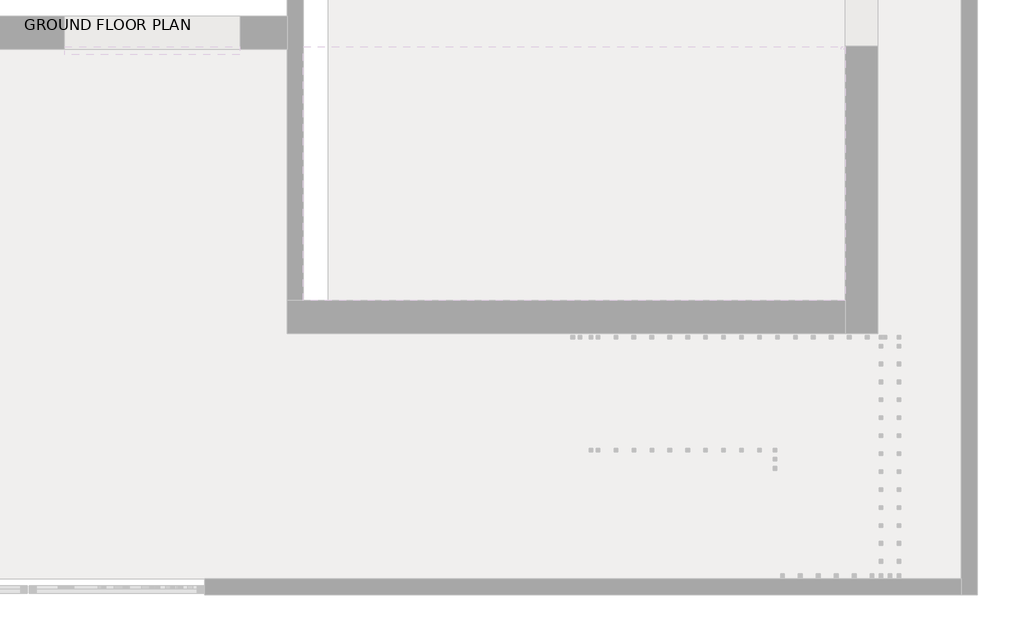
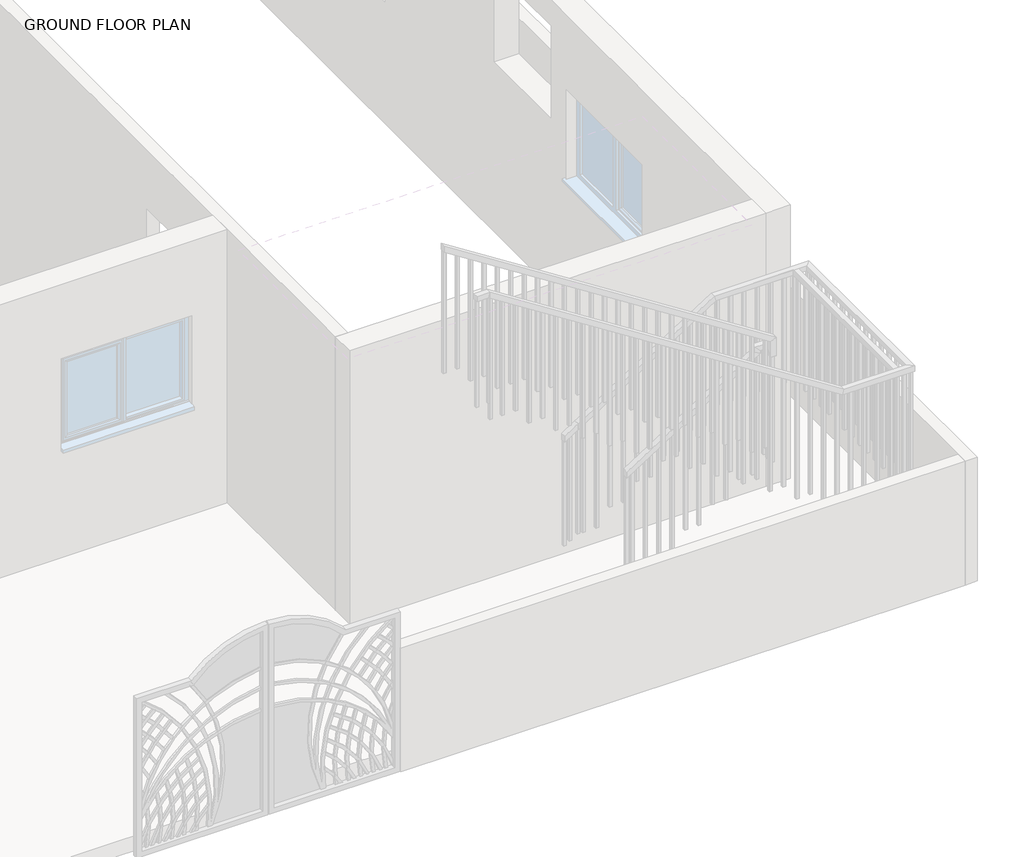
# One storey, part 5 of 23: 2 railings.
"""IFC4 building model written with IfcOpenShell, lengths in millimetres."""

from ifc_helpers import new_model, si_unit, frame, origin, place, context, project, spatial, polyline, outline, extrude, faceted_brep, element, save

model = new_model("IFC4")

# Units and contexts
model_context = context("Model", 3, world=origin())
ifc_project = project(units=[si_unit("LENGTHUNIT", "METRE", prefix="MILLI")], contexts=[model_context])

# Site, building, storey
site = spatial("IfcSite", under=ifc_project)
building = spatial("IfcBuilding", under=site)
storey = spatial("IfcBuildingStorey", under=building, Name="GROUND FLOOR PLAN", Elevation=487.68)

# Railings
placement = place(None, origin())
element("IfcRailing", 1, ObjectType="1100mm", at=placement, inside=storey, context=model_context, shape_type="SolidModel", body=[
    faceted_brep([(-8680.149573, -10220.0521308, 1912.8), (-8680.149573, -10220.0521308, 1853.4423995), (-8680.149573, -10270.0521308, 1853.4423995), (-8680.149573, -10270.0521308, 1912.8), (-7409.7306254, -10220.0521308, 2725.6), (-7395.1045513, -10220.0521308, 2675.6), (-7395.1045513, -10270.0521308, 2675.6), (-7409.7306254, -10270.0521308, 2725.6), (-6495.8132565, -10220.0521308, 2725.6), (-6495.8132565, -10220.0521308, 2675.6), (-6545.8132565, -10270.0521308, 2675.6), (-6545.8132565, -10270.0521308, 2725.6), (-6495.8132565, -11933.6860066, 2725.6), (-6495.8132565, -11933.6860066, 2675.6), (-6545.8132565, -11883.6860066, 2675.6), (-6545.8132565, -11883.6860066, 2725.6), (-7155.718398, -11933.6860066, 2725.6), (-7170.3479429, -11933.6860066, 2675.6), (-7170.3479429, -11883.6860066, 2675.6), (-7155.718398, -11883.6860066, 2725.6), (-10457.8773536, -11933.6860066, 4838.88), (-10457.8773536, -11883.6860066, 4838.88), (-10457.8773536, -11883.6860066, 4779.517542), (-10457.8773536, -11933.6860066, 4779.517542)], [[[0, 1, 2, 3]], [[1, 0, 4, 5]], [[2, 1, 5, 6]], [[3, 2, 6, 7]], [[0, 3, 7, 4]], [[5, 4, 8, 9]], [[6, 5, 9, 10]], [[7, 6, 10, 11]], [[4, 7, 11, 8]], [[9, 8, 12, 13]], [[10, 9, 13, 14]], [[11, 10, 14, 15]], [[8, 11, 15, 12]], [[13, 12, 16, 17]], [[14, 13, 17, 18]], [[15, 14, 18, 19]], [[12, 15, 19, 16]], [[20, 21, 22, 23]], [[17, 16, 20, 23]], [[18, 17, 23, 22]], [[19, 18, 22, 21]], [[16, 19, 21, 20]]]),
    extrude(outline(polyline([(4691.8007425, -10320.8132565), (4707.7999723, -10345.8132565), (3576.32, -10345.8132565), (3576.32, -10320.8132565), (4691.8007425, -10320.8132565)])), frame((0.0, -11921.1860066, 0.0), z_axis=(0.0, 1.0, 0.0), x_axis=(0.0, 0.0, 1.0)), (0.0, 0.0, 1.0), 25.0),
    extrude(outline(polyline([(4611.8045935, -10195.8132565), (4627.8038233, -10220.8132565), (3576.32, -10220.8132565), (3576.32, -10195.8132565), (4611.8045935, -10195.8132565)])), frame((0.0, -11921.1860066, 0.0), z_axis=(0.0, 1.0, 0.0), x_axis=(0.0, 0.0, 1.0)), (0.0, 0.0, 1.0), 25.0),
    extrude(outline(polyline([(4531.8084444, -10070.8132565), (4547.8076742, -10095.8132565), (3413.76, -10095.8132565), (3413.76, -10070.8132565), (4531.8084444, -10070.8132565)])), frame((0.0, -11921.1860066, 0.0), z_axis=(0.0, 1.0, 0.0), x_axis=(0.0, 0.0, 1.0)), (0.0, 0.0, 1.0), 25.0),
    extrude(outline(polyline([(4451.8122954, -9945.8132565), (4467.8115252, -9970.8132565), (3413.76, -9970.8132565), (3413.76, -9945.8132565), (4451.8122954, -9945.8132565)])), frame((0.0, -11921.1860066, 0.0), z_axis=(0.0, 1.0, 0.0), x_axis=(0.0, 0.0, 1.0)), (0.0, 0.0, 1.0), 25.0),
    extrude(outline(polyline([(4371.8161463, -9820.8132565), (4387.8153761, -9845.8132565), (3251.2, -9845.8132565), (3251.2, -9820.8132565), (4371.8161463, -9820.8132565)])), frame((0.0, -11921.1860066, 0.0), z_axis=(0.0, 1.0, 0.0), x_axis=(0.0, 0.0, 1.0)), (0.0, 0.0, 1.0), 25.0),
    extrude(outline(polyline([(4291.8423995, -9695.8132565), (4307.8371231, -9720.8132565), (3251.2, -9720.8132565), (3251.2, -9695.8132565), (4291.8423995, -9695.8132565)])), frame((0.0, -11921.1860066, 0.0), z_axis=(0.0, 1.0, 0.0), x_axis=(0.0, 0.0, 1.0)), (0.0, 0.0, 1.0), 25.0),
    extrude(outline(polyline([(4211.8238482, -9570.8132565), (4227.823078, -9595.8132565), (3088.64, -9595.8132565), (3088.64, -9570.8132565), (4211.8238482, -9570.8132565)])), frame((0.0, -11921.1860066, 0.0), z_axis=(0.0, 1.0, 0.0), x_axis=(0.0, 0.0, 1.0)), (0.0, 0.0, 1.0), 25.0),
    extrude(outline(polyline([(4131.8276992, -9445.8132565), (4147.826929, -9470.8132565), (3088.64, -9470.8132565), (3088.64, -9445.8132565), (4131.8276992, -9445.8132565)])), frame((0.0, -11921.1860066, 0.0), z_axis=(0.0, 1.0, 0.0), x_axis=(0.0, 0.0, 1.0)), (0.0, 0.0, 1.0), 25.0),
    extrude(outline(polyline([(4051.8315501, -9320.8132565), (4067.8307799, -9345.8132565), (2926.08, -9345.8132565), (2926.08, -9320.8132565), (4051.8315501, -9320.8132565)])), frame((0.0, -11921.1860066, 0.0), z_axis=(0.0, 1.0, 0.0), x_axis=(0.0, 0.0, 1.0)), (0.0, 0.0, 1.0), 25.0),
    extrude(outline(polyline([(3971.835401, -9195.8132565), (3987.8346309, -9220.8132565), (2926.08, -9220.8132565), (2926.08, -9195.8132565), (3971.835401, -9195.8132565)])), frame((0.0, -11921.1860066, 0.0), z_axis=(0.0, 1.0, 0.0), x_axis=(0.0, 0.0, 1.0)), (0.0, 0.0, 1.0), 25.0),
    extrude(outline(polyline([(3891.839252, -9070.8132565), (3907.8384818, -9095.8132565), (2763.52, -9095.8132565), (2763.52, -9070.8132565), (3891.839252, -9070.8132565)])), frame((0.0, -11921.1860066, 0.0), z_axis=(0.0, 1.0, 0.0), x_axis=(0.0, 0.0, 1.0)), (0.0, 0.0, 1.0), 25.0),
    extrude(outline(polyline([(3811.8431029, -8945.8132565), (3827.8423328, -8970.8132565), (2763.52, -8970.8132565), (2763.52, -8945.8132565), (3811.8431029, -8945.8132565)])), frame((0.0, -11921.1860066, 0.0), z_axis=(0.0, 1.0, 0.0), x_axis=(0.0, 0.0, 1.0)), (0.0, 0.0, 1.0), 25.0),
    extrude(outline(polyline([(3731.8469539, -8820.8132565), (3747.8461837, -8845.8132565), (2600.96, -8845.8132565), (2600.96, -8820.8132565), (3731.8469539, -8820.8132565)])), frame((0.0, -11921.1860066, 0.0), z_axis=(0.0, 1.0, 0.0), x_axis=(0.0, 0.0, 1.0)), (0.0, 0.0, 1.0), 25.0),
    extrude(outline(polyline([(3651.8508048, -8695.8132565), (3667.8500347, -8720.8132565), (2600.96, -8720.8132565), (2600.96, -8695.8132565), (3651.8508048, -8695.8132565)])), frame((0.0, -11921.1860066, 0.0), z_axis=(0.0, 1.0, 0.0), x_axis=(0.0, 0.0, 1.0)), (0.0, 0.0, 1.0), 25.0),
    extrude(outline(polyline([(3571.8546558, -8570.8132565), (3587.8538856, -8595.8132565), (2438.4, -8595.8132565), (2438.4, -8570.8132565), (3571.8546558, -8570.8132565)])), frame((0.0, -11921.1860066, 0.0), z_axis=(0.0, 1.0, 0.0), x_axis=(0.0, 0.0, 1.0)), (0.0, 0.0, 1.0), 25.0),
    extrude(outline(polyline([(3491.8585067, -8445.8132565), (3507.8577365, -8470.8132565), (2438.4, -8470.8132565), (2438.4, -8445.8132565), (3491.8585067, -8445.8132565)])), frame((0.0, -11921.1860066, 0.0), z_axis=(0.0, 1.0, 0.0), x_axis=(0.0, 0.0, 1.0)), (0.0, 0.0, 1.0), 25.0),
    extrude(outline(polyline([(3411.8623577, -8320.8132565), (3427.8615875, -8345.8132565), (2275.84, -8345.8132565), (2275.84, -8320.8132565), (3411.8623577, -8320.8132565)])), frame((0.0, -11921.1860066, 0.0), z_axis=(0.0, 1.0, 0.0), x_axis=(0.0, 0.0, 1.0)), (0.0, 0.0, 1.0), 25.0),
    extrude(outline(polyline([(3331.8662086, -8195.8132565), (3347.8654384, -8220.8132565), (2275.84, -8220.8132565), (2275.84, -8195.8132565), (3331.8662086, -8195.8132565)])), frame((0.0, -11921.1860066, 0.0), z_axis=(0.0, 1.0, 0.0), x_axis=(0.0, 0.0, 1.0)), (0.0, 0.0, 1.0), 25.0),
    extrude(outline(polyline([(3251.8700596, -8070.8132565), (3267.8692894, -8095.8132565), (2113.28, -8095.8132565), (2113.28, -8070.8132565), (3251.8700596, -8070.8132565)])), frame((0.0, -11921.1860066, 0.0), z_axis=(0.0, 1.0, 0.0), x_axis=(0.0, 0.0, 1.0)), (0.0, 0.0, 1.0), 25.0),
    extrude(outline(polyline([(3171.8739105, -7945.8132565), (3187.8731403, -7970.8132565), (2113.28, -7970.8132565), (2113.28, -7945.8132565), (3171.8739105, -7945.8132565)])), frame((0.0, -11921.1860066, 0.0), z_axis=(0.0, 1.0, 0.0), x_axis=(0.0, 0.0, 1.0)), (0.0, 0.0, 1.0), 25.0),
    extrude(outline(polyline([(3091.8777615, -7820.8132565), (3107.8769913, -7845.8132565), (1950.72, -7845.8132565), (1950.72, -7820.8132565), (3091.8777615, -7820.8132565)])), frame((0.0, -11921.1860066, 0.0), z_axis=(0.0, 1.0, 0.0), x_axis=(0.0, 0.0, 1.0)), (0.0, 0.0, 1.0), 25.0),
    extrude(outline(polyline([(3011.8816124, -7695.8132565), (3027.8808422, -7720.8132565), (1950.72, -7720.8132565), (1950.72, -7695.8132565), (3011.8816124, -7695.8132565)])), frame((0.0, -11921.1860066, 0.0), z_axis=(0.0, 1.0, 0.0), x_axis=(0.0, 0.0, 1.0)), (0.0, 0.0, 1.0), 25.0),
    extrude(outline(polyline([(2931.8854634, -7570.8132565), (2947.8846932, -7595.8132565), (1788.16, -7595.8132565), (1788.16, -7570.8132565), (2931.8854634, -7570.8132565)])), frame((0.0, -11921.1860066, 0.0), z_axis=(0.0, 1.0, 0.0), x_axis=(0.0, 0.0, 1.0)), (0.0, 0.0, 1.0), 25.0),
    extrude(outline(polyline([(2851.8893143, -7445.8132565), (2867.8885441, -7470.8132565), (1788.16, -7470.8132565), (1788.16, -7445.8132565), (2851.8893143, -7445.8132565)])), frame((0.0, -11921.1860066, 0.0), z_axis=(0.0, 1.0, 0.0), x_axis=(0.0, 0.0, 1.0)), (0.0, 0.0, 1.0), 25.0),
    extrude(outline(polyline([(2771.8931653, -7320.8132565), (2787.8923951, -7345.8132565), (1625.6, -7345.8132565), (1625.6, -7320.8132565), (2771.8931653, -7320.8132565)])), frame((0.0, -11921.1860066, 0.0), z_axis=(0.0, 1.0, 0.0), x_axis=(0.0, 0.0, 1.0)), (0.0, 0.0, 1.0), 25.0),
    extrude(outline(polyline([(2691.8970162, -7195.8132565), (2707.896246, -7220.8132565), (1625.6, -7220.8132565), (1625.6, -7195.8132565), (2691.8970162, -7195.8132565)])), frame((0.0, -11921.1860066, 0.0), z_axis=(0.0, 1.0, 0.0), x_axis=(0.0, 0.0, 1.0)), (0.0, 0.0, 1.0), 25.0),
    extrude(outline(polyline([(-7070.8132565, -11921.1860066), (-7095.8132565, -11921.1860066), (-7095.8132565, -11896.1860066), (-7070.8132565, -11896.1860066), (-7070.8132565, -11921.1860066)])), frame((0.0, 0.0, 1625.6), z_axis=(0.0, 0.0, 1.0), x_axis=(1.0, 0.0, 0.0)), (0.0, 0.0, 1.0), 1050.0),
    extrude(outline(polyline([(-6945.8132565, -11921.1860066), (-6970.8132565, -11921.1860066), (-6970.8132565, -11896.1860066), (-6945.8132565, -11896.1860066), (-6945.8132565, -11921.1860066)])), frame((0.0, 0.0, 1625.6), z_axis=(0.0, 0.0, 1.0), x_axis=(1.0, 0.0, 0.0)), (0.0, 0.0, 1.0), 1050.0),
    extrude(outline(polyline([(-6820.8132565, -11921.1860066), (-6845.8132565, -11921.1860066), (-6845.8132565, -11896.1860066), (-6820.8132565, -11896.1860066), (-6820.8132565, -11921.1860066)])), frame((0.0, 0.0, 1625.6), z_axis=(0.0, 0.0, 1.0), x_axis=(1.0, 0.0, 0.0)), (0.0, 0.0, 1.0), 1050.0),
    extrude(outline(polyline([(-6695.8132565, -11921.1860066), (-6720.8132565, -11921.1860066), (-6720.8132565, -11896.1860066), (-6695.8132565, -11896.1860066), (-6695.8132565, -11921.1860066)])), frame((0.0, 0.0, 1625.6), z_axis=(0.0, 0.0, 1.0), x_axis=(1.0, 0.0, 0.0)), (0.0, 0.0, 1.0), 1050.0),
    extrude(outline(polyline([(-6570.8132565, -11921.1860066), (-6595.8132565, -11921.1860066), (-6595.8132565, -11896.1860066), (-6570.8132565, -11896.1860066), (-6570.8132565, -11921.1860066)])), frame((0.0, 0.0, 1625.6), z_axis=(0.0, 0.0, 1.0), x_axis=(1.0, 0.0, 0.0)), (0.0, 0.0, 1.0), 1050.0),
    extrude(outline(polyline([(-6508.3132565, -11795.0521308), (-6508.3132565, -11820.0521308), (-6533.3132565, -11820.0521308), (-6533.3132565, -11795.0521308), (-6508.3132565, -11795.0521308)])), frame((0.0, 0.0, 1625.6), z_axis=(0.0, 0.0, 1.0), x_axis=(1.0, 0.0, 0.0)), (0.0, 0.0, 1.0), 1050.0),
    extrude(outline(polyline([(-6508.3132565, -11670.0521308), (-6508.3132565, -11695.0521308), (-6533.3132565, -11695.0521308), (-6533.3132565, -11670.0521308), (-6508.3132565, -11670.0521308)])), frame((0.0, 0.0, 1625.6), z_axis=(0.0, 0.0, 1.0), x_axis=(1.0, 0.0, 0.0)), (0.0, 0.0, 1.0), 1050.0),
    extrude(outline(polyline([(-6508.3132565, -11545.0521308), (-6508.3132565, -11570.0521308), (-6533.3132565, -11570.0521308), (-6533.3132565, -11545.0521308), (-6508.3132565, -11545.0521308)])), frame((0.0, 0.0, 1625.6), z_axis=(0.0, 0.0, 1.0), x_axis=(1.0, 0.0, 0.0)), (0.0, 0.0, 1.0), 1050.0),
    extrude(outline(polyline([(-6508.3132565, -11420.0521308), (-6508.3132565, -11445.0521308), (-6533.3132565, -11445.0521308), (-6533.3132565, -11420.0521308), (-6508.3132565, -11420.0521308)])), frame((0.0, 0.0, 1625.6), z_axis=(0.0, 0.0, 1.0), x_axis=(1.0, 0.0, 0.0)), (0.0, 0.0, 1.0), 1050.0),
    extrude(outline(polyline([(-6508.3132565, -11295.0521308), (-6508.3132565, -11320.0521308), (-6533.3132565, -11320.0521308), (-6533.3132565, -11295.0521308), (-6508.3132565, -11295.0521308)])), frame((0.0, 0.0, 1625.6), z_axis=(0.0, 0.0, 1.0), x_axis=(1.0, 0.0, 0.0)), (0.0, 0.0, 1.0), 1050.0),
    extrude(outline(polyline([(-6508.3132565, -11170.0521308), (-6508.3132565, -11195.0521308), (-6533.3132565, -11195.0521308), (-6533.3132565, -11170.0521308), (-6508.3132565, -11170.0521308)])), frame((0.0, 0.0, 1625.6), z_axis=(0.0, 0.0, 1.0), x_axis=(1.0, 0.0, 0.0)), (0.0, 0.0, 1.0), 1050.0),
    extrude(outline(polyline([(-6508.3132565, -11045.0521308), (-6508.3132565, -11070.0521308), (-6533.3132565, -11070.0521308), (-6533.3132565, -11045.0521308), (-6508.3132565, -11045.0521308)])), frame((0.0, 0.0, 1625.6), z_axis=(0.0, 0.0, 1.0), x_axis=(1.0, 0.0, 0.0)), (0.0, 0.0, 1.0), 1050.0),
    extrude(outline(polyline([(-6508.3132565, -10920.0521308), (-6508.3132565, -10945.0521308), (-6533.3132565, -10945.0521308), (-6533.3132565, -10920.0521308), (-6508.3132565, -10920.0521308)])), frame((0.0, 0.0, 1625.6), z_axis=(0.0, 0.0, 1.0), x_axis=(1.0, 0.0, 0.0)), (0.0, 0.0, 1.0), 1050.0),
    extrude(outline(polyline([(-6508.3132565, -10795.0521308), (-6508.3132565, -10820.0521308), (-6533.3132565, -10820.0521308), (-6533.3132565, -10795.0521308), (-6508.3132565, -10795.0521308)])), frame((0.0, 0.0, 1625.6), z_axis=(0.0, 0.0, 1.0), x_axis=(1.0, 0.0, 0.0)), (0.0, 0.0, 1.0), 1050.0),
    extrude(outline(polyline([(-6508.3132565, -10670.0521308), (-6508.3132565, -10695.0521308), (-6533.3132565, -10695.0521308), (-6533.3132565, -10670.0521308), (-6508.3132565, -10670.0521308)])), frame((0.0, 0.0, 1625.6), z_axis=(0.0, 0.0, 1.0), x_axis=(1.0, 0.0, 0.0)), (0.0, 0.0, 1.0), 1050.0),
    extrude(outline(polyline([(-6508.3132565, -10545.0521308), (-6508.3132565, -10570.0521308), (-6533.3132565, -10570.0521308), (-6533.3132565, -10545.0521308), (-6508.3132565, -10545.0521308)])), frame((0.0, 0.0, 1625.6), z_axis=(0.0, 0.0, 1.0), x_axis=(1.0, 0.0, 0.0)), (0.0, 0.0, 1.0), 1050.0),
    extrude(outline(polyline([(-6508.3132565, -10420.0521308), (-6508.3132565, -10445.0521308), (-6533.3132565, -10445.0521308), (-6533.3132565, -10420.0521308), (-6508.3132565, -10420.0521308)])), frame((0.0, 0.0, 1625.6), z_axis=(0.0, 0.0, 1.0), x_axis=(1.0, 0.0, 0.0)), (0.0, 0.0, 1.0), 1050.0),
    extrude(outline(polyline([(-6508.3132565, -10295.0521308), (-6508.3132565, -10320.0521308), (-6533.3132565, -10320.0521308), (-6533.3132565, -10295.0521308), (-6508.3132565, -10295.0521308)])), frame((0.0, 0.0, 1625.6), z_axis=(0.0, 0.0, 1.0), x_axis=(1.0, 0.0, 0.0)), (0.0, 0.0, 1.0), 1050.0),
    extrude(outline(polyline([(-6630.149573, -10232.5521308), (-6605.149573, -10232.5521308), (-6605.149573, -10257.5521308), (-6630.149573, -10257.5521308), (-6630.149573, -10232.5521308)])), frame((0.0, 0.0, 1625.6), z_axis=(0.0, 0.0, 1.0), x_axis=(1.0, 0.0, 0.0)), (0.0, 0.0, 1.0), 1050.0),
    extrude(outline(polyline([(-6755.149573, -10232.5521308), (-6730.149573, -10232.5521308), (-6730.149573, -10257.5521308), (-6755.149573, -10257.5521308), (-6755.149573, -10232.5521308)])), frame((0.0, 0.0, 1625.6), z_axis=(0.0, 0.0, 1.0), x_axis=(1.0, 0.0, 0.0)), (0.0, 0.0, 1.0), 1050.0),
    extrude(outline(polyline([(-6880.149573, -10232.5521308), (-6855.149573, -10232.5521308), (-6855.149573, -10257.5521308), (-6880.149573, -10257.5521308), (-6880.149573, -10232.5521308)])), frame((0.0, 0.0, 1625.6), z_axis=(0.0, 0.0, 1.0), x_axis=(1.0, 0.0, 0.0)), (0.0, 0.0, 1.0), 1050.0),
    extrude(outline(polyline([(-7005.149573, -10232.5521308), (-6980.149573, -10232.5521308), (-6980.149573, -10257.5521308), (-7005.149573, -10257.5521308), (-7005.149573, -10232.5521308)])), frame((0.0, 0.0, 1625.6), z_axis=(0.0, 0.0, 1.0), x_axis=(1.0, 0.0, 0.0)), (0.0, 0.0, 1.0), 1050.0),
    extrude(outline(polyline([(-7130.149573, -10232.5521308), (-7105.149573, -10232.5521308), (-7105.149573, -10257.5521308), (-7130.149573, -10257.5521308), (-7130.149573, -10232.5521308)])), frame((0.0, 0.0, 1625.6), z_axis=(0.0, 0.0, 1.0), x_axis=(1.0, 0.0, 0.0)), (0.0, 0.0, 1.0), 1050.0),
    extrude(outline(polyline([(-7255.149573, -10232.5521308), (-7230.149573, -10232.5521308), (-7230.149573, -10257.5521308), (-7255.149573, -10257.5521308), (-7255.149573, -10232.5521308)])), frame((0.0, 0.0, 1625.6), z_axis=(0.0, 0.0, 1.0), x_axis=(1.0, 0.0, 0.0)), (0.0, 0.0, 1.0), 1050.0),
    extrude(outline(polyline([(-7380.149573, -10232.5521308), (-7355.149573, -10232.5521308), (-7355.149573, -10257.5521308), (-7380.149573, -10257.5521308), (-7380.149573, -10232.5521308)])), frame((0.0, 0.0, 1625.6), z_axis=(0.0, 0.0, 1.0), x_axis=(1.0, 0.0, 0.0)), (0.0, 0.0, 1.0), 1050.0),
    extrude(outline(polyline([(1463.04, -7505.149573), (1463.04, -7480.149573), (2621.1891352, -7480.149573), (2605.1944115, -7505.149573), (1463.04, -7505.149573)])), frame((0.0, -10257.5521308, 0.0), z_axis=(0.0, 1.0, 0.0), x_axis=(0.0, 0.0, 1.0)), (0.0, 0.0, 1.0), 25.0),
    extrude(outline(polyline([(1463.04, -7630.149573), (1463.04, -7605.149573), (2541.2155169, -7605.149573), (2525.2207932, -7630.149573), (1463.04, -7630.149573)])), frame((0.0, -10257.5521308, 0.0), z_axis=(0.0, 1.0, 0.0), x_axis=(0.0, 0.0, 1.0)), (0.0, 0.0, 1.0), 25.0),
    extrude(outline(polyline([(1300.48, -7755.149573), (1300.48, -7730.149573), (2461.2418986, -7730.149573), (2445.2471749, -7755.149573), (1300.48, -7755.149573)])), frame((0.0, -10257.5521308, 0.0), z_axis=(0.0, 1.0, 0.0), x_axis=(0.0, 0.0, 1.0)), (0.0, 0.0, 1.0), 25.0),
    extrude(outline(polyline([(1300.48, -7880.149573), (1300.48, -7855.149573), (2381.2682803, -7855.149573), (2365.2735566, -7880.149573), (1300.48, -7880.149573)])), frame((0.0, -10257.5521308, 0.0), z_axis=(0.0, 1.0, 0.0), x_axis=(0.0, 0.0, 1.0)), (0.0, 0.0, 1.0), 25.0),
    extrude(outline(polyline([(1137.92, -8005.149573), (1137.92, -7980.149573), (2301.294662, -7980.149573), (2285.2999383, -8005.149573), (1137.92, -8005.149573)])), frame((0.0, -10257.5521308, 0.0), z_axis=(0.0, 1.0, 0.0), x_axis=(0.0, 0.0, 1.0)), (0.0, 0.0, 1.0), 25.0),
    extrude(outline(polyline([(1137.92, -8130.149573), (1137.92, -8105.149573), (2221.3210437, -8105.149573), (2205.32632, -8130.149573), (1137.92, -8130.149573)])), frame((0.0, -10257.5521308, 0.0), z_axis=(0.0, 1.0, 0.0), x_axis=(0.0, 0.0, 1.0)), (0.0, 0.0, 1.0), 25.0),
    extrude(outline(polyline([(975.36, -8255.149573), (975.36, -8230.149573), (2141.3474254, -8230.149573), (2125.3527017, -8255.149573), (975.36, -8255.149573)])), frame((0.0, -10257.5521308, 0.0), z_axis=(0.0, 1.0, 0.0), x_axis=(0.0, 0.0, 1.0)), (0.0, 0.0, 1.0), 25.0),
    extrude(outline(polyline([(975.36, -8380.149573), (975.36, -8355.149573), (2061.3738071, -8355.149573), (2045.3790834, -8380.149573), (975.36, -8380.149573)])), frame((0.0, -10257.5521308, 0.0), z_axis=(0.0, 1.0, 0.0), x_axis=(0.0, 0.0, 1.0)), (0.0, 0.0, 1.0), 25.0),
    extrude(outline(polyline([(812.8, -8505.149573), (812.8, -8480.149573), (1981.4001888, -8480.149573), (1965.4054651, -8505.149573), (812.8, -8505.149573)])), frame((0.0, -10257.5521308, 0.0), z_axis=(0.0, 1.0, 0.0), x_axis=(0.0, 0.0, 1.0)), (0.0, 0.0, 1.0), 25.0),
    extrude(outline(polyline([(812.8, -8630.149573), (812.8, -8605.149573), (1901.4265705, -8605.149573), (1885.4318468, -8630.149573), (812.8, -8630.149573)])), frame((0.0, -10257.5521308, 0.0), z_axis=(0.0, 1.0, 0.0), x_axis=(0.0, 0.0, 1.0)), (0.0, 0.0, 1.0), 25.0),
    extrude(outline(polyline([(-6508.3132565, -11896.1860066), (-6508.3132565, -11921.1860066), (-6533.3132565, -11921.1860066), (-6533.3132565, -11896.1860066), (-6508.3132565, -11896.1860066)])), frame((0.0, 0.0, 1625.6), z_axis=(0.0, 0.0, 1.0), x_axis=(1.0, 0.0, 0.0)), (0.0, 0.0, 1.0), 1050.0),
    extrude(outline(polyline([(-6533.3132565, -10232.5521308), (-6508.3132565, -10232.5521308), (-6508.3132565, -10257.5521308), (-6533.3132565, -10257.5521308), (-6533.3132565, -10232.5521308)])), frame((0.0, 0.0, 1625.6), z_axis=(0.0, 0.0, 1.0), x_axis=(1.0, 0.0, 0.0)), (0.0, 0.0, 1.0), 1050.0),
    extrude(outline(polyline([(4763.5183122, -10432.8773536), (4779.517542, -10457.8773536), (3576.32, -10457.8773536), (3576.32, -10432.8773536), (4763.5183122, -10432.8773536)])), frame((0.0, -11921.1860066, 0.0), z_axis=(0.0, 1.0, 0.0), x_axis=(0.0, 0.0, 1.0)), (0.0, 0.0, 1.0), 25.0),
    extrude(outline(polyline([(812.8, -8680.149573), (812.8, -8655.149573), (1869.4371231, -8655.149573), (1853.4423995, -8680.149573), (812.8, -8680.149573)])), frame((0.0, -10257.5521308, 0.0), z_axis=(0.0, 1.0, 0.0), x_axis=(0.0, 0.0, 1.0)), (0.0, 0.0, 1.0), 25.0),
])
element("IfcRailing", 2, ObjectType="1100mm", at=placement, inside=storey, context=model_context, shape_type="SolidModel", body=[
    faceted_brep([(-8680.149573, -10220.0521308, 1912.8), (-8680.149573, -10220.0521308, 1853.4423995), (-8680.149573, -10270.0521308, 1853.4423995), (-8680.149573, -10270.0521308, 1912.8), (-7409.7306254, -10220.0521308, 2725.6), (-7395.1045513, -10220.0521308, 2675.6), (-7395.1045513, -10270.0521308, 2675.6), (-7409.7306254, -10270.0521308, 2725.6), (-6495.8132565, -10220.0521308, 2725.6), (-6495.8132565, -10220.0521308, 2675.6), (-6545.8132565, -10270.0521308, 2675.6), (-6545.8132565, -10270.0521308, 2725.6), (-6495.8132565, -11933.6860066, 2725.6), (-6495.8132565, -11933.6860066, 2675.6), (-6545.8132565, -11883.6860066, 2675.6), (-6545.8132565, -11883.6860066, 2725.6), (-7155.718398, -11933.6860066, 2725.6), (-7170.3479429, -11933.6860066, 2675.6), (-7170.3479429, -11883.6860066, 2675.6), (-7155.718398, -11883.6860066, 2725.6), (-10457.8773536, -11933.6860066, 4838.88), (-10457.8773536, -11883.6860066, 4838.88), (-10457.8773536, -11883.6860066, 4779.517542), (-10457.8773536, -11933.6860066, 4779.517542)], [[[0, 1, 2, 3]], [[1, 0, 4, 5]], [[2, 1, 5, 6]], [[3, 2, 6, 7]], [[0, 3, 7, 4]], [[5, 4, 8, 9]], [[6, 5, 9, 10]], [[7, 6, 10, 11]], [[4, 7, 11, 8]], [[9, 8, 12, 13]], [[10, 9, 13, 14]], [[11, 10, 14, 15]], [[8, 11, 15, 12]], [[13, 12, 16, 17]], [[14, 13, 17, 18]], [[15, 14, 18, 19]], [[12, 15, 19, 16]], [[20, 21, 22, 23]], [[17, 16, 20, 23]], [[18, 17, 23, 22]], [[19, 18, 22, 21]], [[16, 19, 21, 20]]]),
    extrude(outline(polyline([(4691.8007425, -10320.8132565), (4707.7999723, -10345.8132565), (3576.32, -10345.8132565), (3576.32, -10320.8132565), (4691.8007425, -10320.8132565)])), frame((0.0, -11921.1860066, 0.0), z_axis=(0.0, 1.0, 0.0), x_axis=(0.0, 0.0, 1.0)), (0.0, 0.0, 1.0), 25.0),
    extrude(outline(polyline([(4611.8045935, -10195.8132565), (4627.8038233, -10220.8132565), (3576.32, -10220.8132565), (3576.32, -10195.8132565), (4611.8045935, -10195.8132565)])), frame((0.0, -11921.1860066, 0.0), z_axis=(0.0, 1.0, 0.0), x_axis=(0.0, 0.0, 1.0)), (0.0, 0.0, 1.0), 25.0),
    extrude(outline(polyline([(4531.8084444, -10070.8132565), (4547.8076742, -10095.8132565), (3413.76, -10095.8132565), (3413.76, -10070.8132565), (4531.8084444, -10070.8132565)])), frame((0.0, -11921.1860066, 0.0), z_axis=(0.0, 1.0, 0.0), x_axis=(0.0, 0.0, 1.0)), (0.0, 0.0, 1.0), 25.0),
    extrude(outline(polyline([(4451.8122954, -9945.8132565), (4467.8115252, -9970.8132565), (3413.76, -9970.8132565), (3413.76, -9945.8132565), (4451.8122954, -9945.8132565)])), frame((0.0, -11921.1860066, 0.0), z_axis=(0.0, 1.0, 0.0), x_axis=(0.0, 0.0, 1.0)), (0.0, 0.0, 1.0), 25.0),
    extrude(outline(polyline([(4371.8161463, -9820.8132565), (4387.8153761, -9845.8132565), (3251.2, -9845.8132565), (3251.2, -9820.8132565), (4371.8161463, -9820.8132565)])), frame((0.0, -11921.1860066, 0.0), z_axis=(0.0, 1.0, 0.0), x_axis=(0.0, 0.0, 1.0)), (0.0, 0.0, 1.0), 25.0),
    extrude(outline(polyline([(4291.8423995, -9695.8132565), (4307.8371231, -9720.8132565), (3251.2, -9720.8132565), (3251.2, -9695.8132565), (4291.8423995, -9695.8132565)])), frame((0.0, -11921.1860066, 0.0), z_axis=(0.0, 1.0, 0.0), x_axis=(0.0, 0.0, 1.0)), (0.0, 0.0, 1.0), 25.0),
    extrude(outline(polyline([(4211.8238482, -9570.8132565), (4227.823078, -9595.8132565), (3088.64, -9595.8132565), (3088.64, -9570.8132565), (4211.8238482, -9570.8132565)])), frame((0.0, -11921.1860066, 0.0), z_axis=(0.0, 1.0, 0.0), x_axis=(0.0, 0.0, 1.0)), (0.0, 0.0, 1.0), 25.0),
    extrude(outline(polyline([(4131.8276992, -9445.8132565), (4147.826929, -9470.8132565), (3088.64, -9470.8132565), (3088.64, -9445.8132565), (4131.8276992, -9445.8132565)])), frame((0.0, -11921.1860066, 0.0), z_axis=(0.0, 1.0, 0.0), x_axis=(0.0, 0.0, 1.0)), (0.0, 0.0, 1.0), 25.0),
    extrude(outline(polyline([(4051.8315501, -9320.8132565), (4067.8307799, -9345.8132565), (2926.08, -9345.8132565), (2926.08, -9320.8132565), (4051.8315501, -9320.8132565)])), frame((0.0, -11921.1860066, 0.0), z_axis=(0.0, 1.0, 0.0), x_axis=(0.0, 0.0, 1.0)), (0.0, 0.0, 1.0), 25.0),
    extrude(outline(polyline([(3971.835401, -9195.8132565), (3987.8346309, -9220.8132565), (2926.08, -9220.8132565), (2926.08, -9195.8132565), (3971.835401, -9195.8132565)])), frame((0.0, -11921.1860066, 0.0), z_axis=(0.0, 1.0, 0.0), x_axis=(0.0, 0.0, 1.0)), (0.0, 0.0, 1.0), 25.0),
    extrude(outline(polyline([(3891.839252, -9070.8132565), (3907.8384818, -9095.8132565), (2763.52, -9095.8132565), (2763.52, -9070.8132565), (3891.839252, -9070.8132565)])), frame((0.0, -11921.1860066, 0.0), z_axis=(0.0, 1.0, 0.0), x_axis=(0.0, 0.0, 1.0)), (0.0, 0.0, 1.0), 25.0),
    extrude(outline(polyline([(3811.8431029, -8945.8132565), (3827.8423328, -8970.8132565), (2763.52, -8970.8132565), (2763.52, -8945.8132565), (3811.8431029, -8945.8132565)])), frame((0.0, -11921.1860066, 0.0), z_axis=(0.0, 1.0, 0.0), x_axis=(0.0, 0.0, 1.0)), (0.0, 0.0, 1.0), 25.0),
    extrude(outline(polyline([(3731.8469539, -8820.8132565), (3747.8461837, -8845.8132565), (2600.96, -8845.8132565), (2600.96, -8820.8132565), (3731.8469539, -8820.8132565)])), frame((0.0, -11921.1860066, 0.0), z_axis=(0.0, 1.0, 0.0), x_axis=(0.0, 0.0, 1.0)), (0.0, 0.0, 1.0), 25.0),
    extrude(outline(polyline([(3651.8508048, -8695.8132565), (3667.8500347, -8720.8132565), (2600.96, -8720.8132565), (2600.96, -8695.8132565), (3651.8508048, -8695.8132565)])), frame((0.0, -11921.1860066, 0.0), z_axis=(0.0, 1.0, 0.0), x_axis=(0.0, 0.0, 1.0)), (0.0, 0.0, 1.0), 25.0),
    extrude(outline(polyline([(3571.8546558, -8570.8132565), (3587.8538856, -8595.8132565), (2438.4, -8595.8132565), (2438.4, -8570.8132565), (3571.8546558, -8570.8132565)])), frame((0.0, -11921.1860066, 0.0), z_axis=(0.0, 1.0, 0.0), x_axis=(0.0, 0.0, 1.0)), (0.0, 0.0, 1.0), 25.0),
    extrude(outline(polyline([(3491.8585067, -8445.8132565), (3507.8577365, -8470.8132565), (2438.4, -8470.8132565), (2438.4, -8445.8132565), (3491.8585067, -8445.8132565)])), frame((0.0, -11921.1860066, 0.0), z_axis=(0.0, 1.0, 0.0), x_axis=(0.0, 0.0, 1.0)), (0.0, 0.0, 1.0), 25.0),
    extrude(outline(polyline([(3411.8623577, -8320.8132565), (3427.8615875, -8345.8132565), (2275.84, -8345.8132565), (2275.84, -8320.8132565), (3411.8623577, -8320.8132565)])), frame((0.0, -11921.1860066, 0.0), z_axis=(0.0, 1.0, 0.0), x_axis=(0.0, 0.0, 1.0)), (0.0, 0.0, 1.0), 25.0),
    extrude(outline(polyline([(3331.8662086, -8195.8132565), (3347.8654384, -8220.8132565), (2275.84, -8220.8132565), (2275.84, -8195.8132565), (3331.8662086, -8195.8132565)])), frame((0.0, -11921.1860066, 0.0), z_axis=(0.0, 1.0, 0.0), x_axis=(0.0, 0.0, 1.0)), (0.0, 0.0, 1.0), 25.0),
    extrude(outline(polyline([(3251.8700596, -8070.8132565), (3267.8692894, -8095.8132565), (2113.28, -8095.8132565), (2113.28, -8070.8132565), (3251.8700596, -8070.8132565)])), frame((0.0, -11921.1860066, 0.0), z_axis=(0.0, 1.0, 0.0), x_axis=(0.0, 0.0, 1.0)), (0.0, 0.0, 1.0), 25.0),
    extrude(outline(polyline([(3171.8739105, -7945.8132565), (3187.8731403, -7970.8132565), (2113.28, -7970.8132565), (2113.28, -7945.8132565), (3171.8739105, -7945.8132565)])), frame((0.0, -11921.1860066, 0.0), z_axis=(0.0, 1.0, 0.0), x_axis=(0.0, 0.0, 1.0)), (0.0, 0.0, 1.0), 25.0),
    extrude(outline(polyline([(3091.8777615, -7820.8132565), (3107.8769913, -7845.8132565), (1950.72, -7845.8132565), (1950.72, -7820.8132565), (3091.8777615, -7820.8132565)])), frame((0.0, -11921.1860066, 0.0), z_axis=(0.0, 1.0, 0.0), x_axis=(0.0, 0.0, 1.0)), (0.0, 0.0, 1.0), 25.0),
    extrude(outline(polyline([(3011.8816124, -7695.8132565), (3027.8808422, -7720.8132565), (1950.72, -7720.8132565), (1950.72, -7695.8132565), (3011.8816124, -7695.8132565)])), frame((0.0, -11921.1860066, 0.0), z_axis=(0.0, 1.0, 0.0), x_axis=(0.0, 0.0, 1.0)), (0.0, 0.0, 1.0), 25.0),
    extrude(outline(polyline([(2931.8854634, -7570.8132565), (2947.8846932, -7595.8132565), (1788.16, -7595.8132565), (1788.16, -7570.8132565), (2931.8854634, -7570.8132565)])), frame((0.0, -11921.1860066, 0.0), z_axis=(0.0, 1.0, 0.0), x_axis=(0.0, 0.0, 1.0)), (0.0, 0.0, 1.0), 25.0),
    extrude(outline(polyline([(2851.8893143, -7445.8132565), (2867.8885441, -7470.8132565), (1788.16, -7470.8132565), (1788.16, -7445.8132565), (2851.8893143, -7445.8132565)])), frame((0.0, -11921.1860066, 0.0), z_axis=(0.0, 1.0, 0.0), x_axis=(0.0, 0.0, 1.0)), (0.0, 0.0, 1.0), 25.0),
    extrude(outline(polyline([(2771.8931653, -7320.8132565), (2787.8923951, -7345.8132565), (1625.6, -7345.8132565), (1625.6, -7320.8132565), (2771.8931653, -7320.8132565)])), frame((0.0, -11921.1860066, 0.0), z_axis=(0.0, 1.0, 0.0), x_axis=(0.0, 0.0, 1.0)), (0.0, 0.0, 1.0), 25.0),
    extrude(outline(polyline([(2691.8970162, -7195.8132565), (2707.896246, -7220.8132565), (1625.6, -7220.8132565), (1625.6, -7195.8132565), (2691.8970162, -7195.8132565)])), frame((0.0, -11921.1860066, 0.0), z_axis=(0.0, 1.0, 0.0), x_axis=(0.0, 0.0, 1.0)), (0.0, 0.0, 1.0), 25.0),
    extrude(outline(polyline([(-7070.8132565, -11921.1860066), (-7095.8132565, -11921.1860066), (-7095.8132565, -11896.1860066), (-7070.8132565, -11896.1860066), (-7070.8132565, -11921.1860066)])), frame((0.0, 0.0, 1625.6), z_axis=(0.0, 0.0, 1.0), x_axis=(1.0, 0.0, 0.0)), (0.0, 0.0, 1.0), 1050.0),
    extrude(outline(polyline([(-6945.8132565, -11921.1860066), (-6970.8132565, -11921.1860066), (-6970.8132565, -11896.1860066), (-6945.8132565, -11896.1860066), (-6945.8132565, -11921.1860066)])), frame((0.0, 0.0, 1625.6), z_axis=(0.0, 0.0, 1.0), x_axis=(1.0, 0.0, 0.0)), (0.0, 0.0, 1.0), 1050.0),
    extrude(outline(polyline([(-6820.8132565, -11921.1860066), (-6845.8132565, -11921.1860066), (-6845.8132565, -11896.1860066), (-6820.8132565, -11896.1860066), (-6820.8132565, -11921.1860066)])), frame((0.0, 0.0, 1625.6), z_axis=(0.0, 0.0, 1.0), x_axis=(1.0, 0.0, 0.0)), (0.0, 0.0, 1.0), 1050.0),
    extrude(outline(polyline([(-6695.8132565, -11921.1860066), (-6720.8132565, -11921.1860066), (-6720.8132565, -11896.1860066), (-6695.8132565, -11896.1860066), (-6695.8132565, -11921.1860066)])), frame((0.0, 0.0, 1625.6), z_axis=(0.0, 0.0, 1.0), x_axis=(1.0, 0.0, 0.0)), (0.0, 0.0, 1.0), 1050.0),
    extrude(outline(polyline([(-6570.8132565, -11921.1860066), (-6595.8132565, -11921.1860066), (-6595.8132565, -11896.1860066), (-6570.8132565, -11896.1860066), (-6570.8132565, -11921.1860066)])), frame((0.0, 0.0, 1625.6), z_axis=(0.0, 0.0, 1.0), x_axis=(1.0, 0.0, 0.0)), (0.0, 0.0, 1.0), 1050.0),
    extrude(outline(polyline([(-6508.3132565, -11795.0521308), (-6508.3132565, -11820.0521308), (-6533.3132565, -11820.0521308), (-6533.3132565, -11795.0521308), (-6508.3132565, -11795.0521308)])), frame((0.0, 0.0, 1625.6), z_axis=(0.0, 0.0, 1.0), x_axis=(1.0, 0.0, 0.0)), (0.0, 0.0, 1.0), 1050.0),
    extrude(outline(polyline([(-6508.3132565, -11670.0521308), (-6508.3132565, -11695.0521308), (-6533.3132565, -11695.0521308), (-6533.3132565, -11670.0521308), (-6508.3132565, -11670.0521308)])), frame((0.0, 0.0, 1625.6), z_axis=(0.0, 0.0, 1.0), x_axis=(1.0, 0.0, 0.0)), (0.0, 0.0, 1.0), 1050.0),
    extrude(outline(polyline([(-6508.3132565, -11545.0521308), (-6508.3132565, -11570.0521308), (-6533.3132565, -11570.0521308), (-6533.3132565, -11545.0521308), (-6508.3132565, -11545.0521308)])), frame((0.0, 0.0, 1625.6), z_axis=(0.0, 0.0, 1.0), x_axis=(1.0, 0.0, 0.0)), (0.0, 0.0, 1.0), 1050.0),
    extrude(outline(polyline([(-6508.3132565, -11420.0521308), (-6508.3132565, -11445.0521308), (-6533.3132565, -11445.0521308), (-6533.3132565, -11420.0521308), (-6508.3132565, -11420.0521308)])), frame((0.0, 0.0, 1625.6), z_axis=(0.0, 0.0, 1.0), x_axis=(1.0, 0.0, 0.0)), (0.0, 0.0, 1.0), 1050.0),
    extrude(outline(polyline([(-6508.3132565, -11295.0521308), (-6508.3132565, -11320.0521308), (-6533.3132565, -11320.0521308), (-6533.3132565, -11295.0521308), (-6508.3132565, -11295.0521308)])), frame((0.0, 0.0, 1625.6), z_axis=(0.0, 0.0, 1.0), x_axis=(1.0, 0.0, 0.0)), (0.0, 0.0, 1.0), 1050.0),
    extrude(outline(polyline([(-6508.3132565, -11170.0521308), (-6508.3132565, -11195.0521308), (-6533.3132565, -11195.0521308), (-6533.3132565, -11170.0521308), (-6508.3132565, -11170.0521308)])), frame((0.0, 0.0, 1625.6), z_axis=(0.0, 0.0, 1.0), x_axis=(1.0, 0.0, 0.0)), (0.0, 0.0, 1.0), 1050.0),
    extrude(outline(polyline([(-6508.3132565, -11045.0521308), (-6508.3132565, -11070.0521308), (-6533.3132565, -11070.0521308), (-6533.3132565, -11045.0521308), (-6508.3132565, -11045.0521308)])), frame((0.0, 0.0, 1625.6), z_axis=(0.0, 0.0, 1.0), x_axis=(1.0, 0.0, 0.0)), (0.0, 0.0, 1.0), 1050.0),
    extrude(outline(polyline([(-6508.3132565, -10920.0521308), (-6508.3132565, -10945.0521308), (-6533.3132565, -10945.0521308), (-6533.3132565, -10920.0521308), (-6508.3132565, -10920.0521308)])), frame((0.0, 0.0, 1625.6), z_axis=(0.0, 0.0, 1.0), x_axis=(1.0, 0.0, 0.0)), (0.0, 0.0, 1.0), 1050.0),
    extrude(outline(polyline([(-6508.3132565, -10795.0521308), (-6508.3132565, -10820.0521308), (-6533.3132565, -10820.0521308), (-6533.3132565, -10795.0521308), (-6508.3132565, -10795.0521308)])), frame((0.0, 0.0, 1625.6), z_axis=(0.0, 0.0, 1.0), x_axis=(1.0, 0.0, 0.0)), (0.0, 0.0, 1.0), 1050.0),
    extrude(outline(polyline([(-6508.3132565, -10670.0521308), (-6508.3132565, -10695.0521308), (-6533.3132565, -10695.0521308), (-6533.3132565, -10670.0521308), (-6508.3132565, -10670.0521308)])), frame((0.0, 0.0, 1625.6), z_axis=(0.0, 0.0, 1.0), x_axis=(1.0, 0.0, 0.0)), (0.0, 0.0, 1.0), 1050.0),
    extrude(outline(polyline([(-6508.3132565, -10545.0521308), (-6508.3132565, -10570.0521308), (-6533.3132565, -10570.0521308), (-6533.3132565, -10545.0521308), (-6508.3132565, -10545.0521308)])), frame((0.0, 0.0, 1625.6), z_axis=(0.0, 0.0, 1.0), x_axis=(1.0, 0.0, 0.0)), (0.0, 0.0, 1.0), 1050.0),
    extrude(outline(polyline([(-6508.3132565, -10420.0521308), (-6508.3132565, -10445.0521308), (-6533.3132565, -10445.0521308), (-6533.3132565, -10420.0521308), (-6508.3132565, -10420.0521308)])), frame((0.0, 0.0, 1625.6), z_axis=(0.0, 0.0, 1.0), x_axis=(1.0, 0.0, 0.0)), (0.0, 0.0, 1.0), 1050.0),
    extrude(outline(polyline([(-6508.3132565, -10295.0521308), (-6508.3132565, -10320.0521308), (-6533.3132565, -10320.0521308), (-6533.3132565, -10295.0521308), (-6508.3132565, -10295.0521308)])), frame((0.0, 0.0, 1625.6), z_axis=(0.0, 0.0, 1.0), x_axis=(1.0, 0.0, 0.0)), (0.0, 0.0, 1.0), 1050.0),
    extrude(outline(polyline([(-6630.149573, -10232.5521308), (-6605.149573, -10232.5521308), (-6605.149573, -10257.5521308), (-6630.149573, -10257.5521308), (-6630.149573, -10232.5521308)])), frame((0.0, 0.0, 1625.6), z_axis=(0.0, 0.0, 1.0), x_axis=(1.0, 0.0, 0.0)), (0.0, 0.0, 1.0), 1050.0),
    extrude(outline(polyline([(-6755.149573, -10232.5521308), (-6730.149573, -10232.5521308), (-6730.149573, -10257.5521308), (-6755.149573, -10257.5521308), (-6755.149573, -10232.5521308)])), frame((0.0, 0.0, 1625.6), z_axis=(0.0, 0.0, 1.0), x_axis=(1.0, 0.0, 0.0)), (0.0, 0.0, 1.0), 1050.0),
    extrude(outline(polyline([(-6880.149573, -10232.5521308), (-6855.149573, -10232.5521308), (-6855.149573, -10257.5521308), (-6880.149573, -10257.5521308), (-6880.149573, -10232.5521308)])), frame((0.0, 0.0, 1625.6), z_axis=(0.0, 0.0, 1.0), x_axis=(1.0, 0.0, 0.0)), (0.0, 0.0, 1.0), 1050.0),
    extrude(outline(polyline([(-7005.149573, -10232.5521308), (-6980.149573, -10232.5521308), (-6980.149573, -10257.5521308), (-7005.149573, -10257.5521308), (-7005.149573, -10232.5521308)])), frame((0.0, 0.0, 1625.6), z_axis=(0.0, 0.0, 1.0), x_axis=(1.0, 0.0, 0.0)), (0.0, 0.0, 1.0), 1050.0),
    extrude(outline(polyline([(-7130.149573, -10232.5521308), (-7105.149573, -10232.5521308), (-7105.149573, -10257.5521308), (-7130.149573, -10257.5521308), (-7130.149573, -10232.5521308)])), frame((0.0, 0.0, 1625.6), z_axis=(0.0, 0.0, 1.0), x_axis=(1.0, 0.0, 0.0)), (0.0, 0.0, 1.0), 1050.0),
    extrude(outline(polyline([(-7255.149573, -10232.5521308), (-7230.149573, -10232.5521308), (-7230.149573, -10257.5521308), (-7255.149573, -10257.5521308), (-7255.149573, -10232.5521308)])), frame((0.0, 0.0, 1625.6), z_axis=(0.0, 0.0, 1.0), x_axis=(1.0, 0.0, 0.0)), (0.0, 0.0, 1.0), 1050.0),
    extrude(outline(polyline([(-7380.149573, -10232.5521308), (-7355.149573, -10232.5521308), (-7355.149573, -10257.5521308), (-7380.149573, -10257.5521308), (-7380.149573, -10232.5521308)])), frame((0.0, 0.0, 1625.6), z_axis=(0.0, 0.0, 1.0), x_axis=(1.0, 0.0, 0.0)), (0.0, 0.0, 1.0), 1050.0),
    extrude(outline(polyline([(1463.04, -7505.149573), (1463.04, -7480.149573), (2621.1891352, -7480.149573), (2605.1944115, -7505.149573), (1463.04, -7505.149573)])), frame((0.0, -10257.5521308, 0.0), z_axis=(0.0, 1.0, 0.0), x_axis=(0.0, 0.0, 1.0)), (0.0, 0.0, 1.0), 25.0),
    extrude(outline(polyline([(1463.04, -7630.149573), (1463.04, -7605.149573), (2541.2155169, -7605.149573), (2525.2207932, -7630.149573), (1463.04, -7630.149573)])), frame((0.0, -10257.5521308, 0.0), z_axis=(0.0, 1.0, 0.0), x_axis=(0.0, 0.0, 1.0)), (0.0, 0.0, 1.0), 25.0),
    extrude(outline(polyline([(1300.48, -7755.149573), (1300.48, -7730.149573), (2461.2418986, -7730.149573), (2445.2471749, -7755.149573), (1300.48, -7755.149573)])), frame((0.0, -10257.5521308, 0.0), z_axis=(0.0, 1.0, 0.0), x_axis=(0.0, 0.0, 1.0)), (0.0, 0.0, 1.0), 25.0),
    extrude(outline(polyline([(1300.48, -7880.149573), (1300.48, -7855.149573), (2381.2682803, -7855.149573), (2365.2735566, -7880.149573), (1300.48, -7880.149573)])), frame((0.0, -10257.5521308, 0.0), z_axis=(0.0, 1.0, 0.0), x_axis=(0.0, 0.0, 1.0)), (0.0, 0.0, 1.0), 25.0),
    extrude(outline(polyline([(1137.92, -8005.149573), (1137.92, -7980.149573), (2301.294662, -7980.149573), (2285.2999383, -8005.149573), (1137.92, -8005.149573)])), frame((0.0, -10257.5521308, 0.0), z_axis=(0.0, 1.0, 0.0), x_axis=(0.0, 0.0, 1.0)), (0.0, 0.0, 1.0), 25.0),
    extrude(outline(polyline([(1137.92, -8130.149573), (1137.92, -8105.149573), (2221.3210437, -8105.149573), (2205.32632, -8130.149573), (1137.92, -8130.149573)])), frame((0.0, -10257.5521308, 0.0), z_axis=(0.0, 1.0, 0.0), x_axis=(0.0, 0.0, 1.0)), (0.0, 0.0, 1.0), 25.0),
    extrude(outline(polyline([(975.36, -8255.149573), (975.36, -8230.149573), (2141.3474254, -8230.149573), (2125.3527017, -8255.149573), (975.36, -8255.149573)])), frame((0.0, -10257.5521308, 0.0), z_axis=(0.0, 1.0, 0.0), x_axis=(0.0, 0.0, 1.0)), (0.0, 0.0, 1.0), 25.0),
    extrude(outline(polyline([(975.36, -8380.149573), (975.36, -8355.149573), (2061.3738071, -8355.149573), (2045.3790834, -8380.149573), (975.36, -8380.149573)])), frame((0.0, -10257.5521308, 0.0), z_axis=(0.0, 1.0, 0.0), x_axis=(0.0, 0.0, 1.0)), (0.0, 0.0, 1.0), 25.0),
    extrude(outline(polyline([(812.8, -8505.149573), (812.8, -8480.149573), (1981.4001888, -8480.149573), (1965.4054651, -8505.149573), (812.8, -8505.149573)])), frame((0.0, -10257.5521308, 0.0), z_axis=(0.0, 1.0, 0.0), x_axis=(0.0, 0.0, 1.0)), (0.0, 0.0, 1.0), 25.0),
    extrude(outline(polyline([(812.8, -8630.149573), (812.8, -8605.149573), (1901.4265705, -8605.149573), (1885.4318468, -8630.149573), (812.8, -8630.149573)])), frame((0.0, -10257.5521308, 0.0), z_axis=(0.0, 1.0, 0.0), x_axis=(0.0, 0.0, 1.0)), (0.0, 0.0, 1.0), 25.0),
    extrude(outline(polyline([(-6508.3132565, -11896.1860066), (-6508.3132565, -11921.1860066), (-6533.3132565, -11921.1860066), (-6533.3132565, -11896.1860066), (-6508.3132565, -11896.1860066)])), frame((0.0, 0.0, 1625.6), z_axis=(0.0, 0.0, 1.0), x_axis=(1.0, 0.0, 0.0)), (0.0, 0.0, 1.0), 1050.0),
    extrude(outline(polyline([(-6533.3132565, -10232.5521308), (-6508.3132565, -10232.5521308), (-6508.3132565, -10257.5521308), (-6533.3132565, -10257.5521308), (-6533.3132565, -10232.5521308)])), frame((0.0, 0.0, 1625.6), z_axis=(0.0, 0.0, 1.0), x_axis=(1.0, 0.0, 0.0)), (0.0, 0.0, 1.0), 1050.0),
    extrude(outline(polyline([(4763.5183122, -10432.8773536), (4779.517542, -10457.8773536), (3576.32, -10457.8773536), (3576.32, -10432.8773536), (4763.5183122, -10432.8773536)])), frame((0.0, -11921.1860066, 0.0), z_axis=(0.0, 1.0, 0.0), x_axis=(0.0, 0.0, 1.0)), (0.0, 0.0, 1.0), 25.0),
    extrude(outline(polyline([(812.8, -8680.149573), (812.8, -8655.149573), (1869.4371231, -8655.149573), (1853.4423995, -8680.149573), (812.8, -8680.149573)])), frame((0.0, -10257.5521308, 0.0), z_axis=(0.0, 1.0, 0.0), x_axis=(0.0, 0.0, 1.0)), (0.0, 0.0, 1.0), 25.0),
])

save(model, "model.ifc")

# Revit data of these elements
# Type "1100mm"
#   built-in parameter 1008612 = 0.019685 (stored number, unit not read)
#   built-in parameter 1008611 = 0.019685 (stored number, unit not read)
#   built-in parameter 1008609 = 0.902231 (stored number, unit not read)
#   built-in parameter 1008604 = 0.19685 (stored number, unit not read)
#   built-in parameter 1008603 = 0.164042 (stored number, unit not read)
#   Railing Height = 3.608924 ft
#   built-in parameter 1008630 = 2
#   built-in parameter 1008610 = 2
#   built-in parameter 1008608 = 1
#   built-in parameter 1008618 = Baluster_Square : 25mm
# Elements 1, 2 (IfcRailing, "1100mm")
#   Phase Created = New Construction
